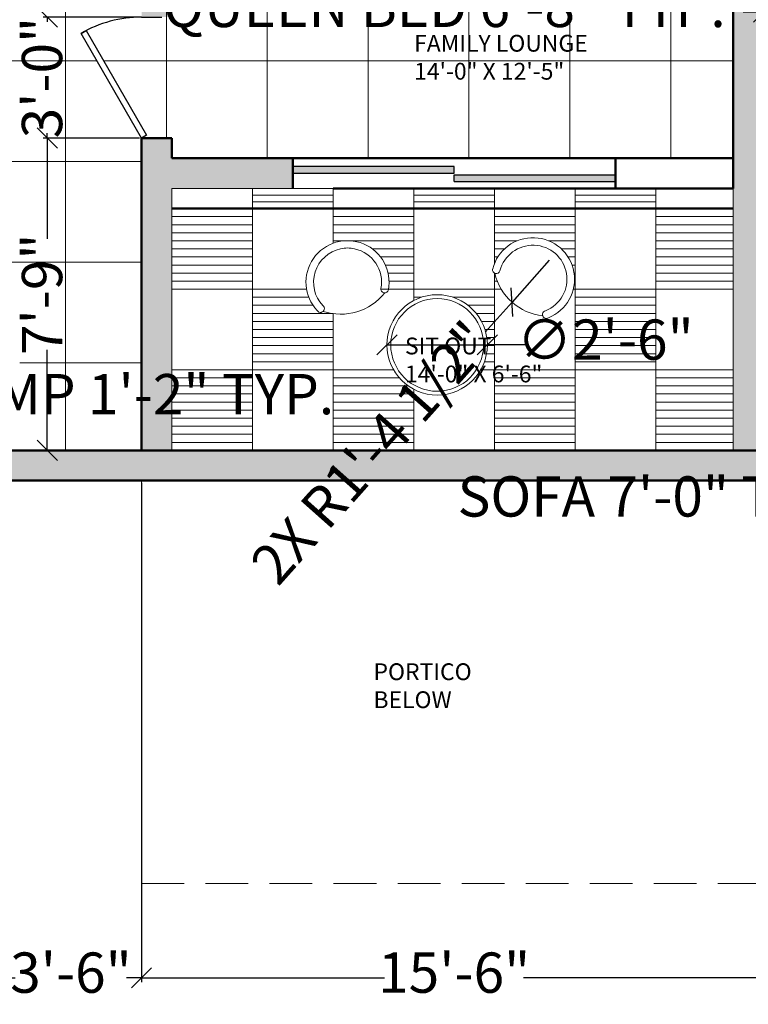
# Model space of a CAD drawing. Units: inches. Extents: x 2371 to 3019, y 129 to 700.
# Tile 2 of 14: x 2536 to 2753, y 139 to 432. Entities that reach past the tile are written whole.
import ezdxf

# ---------------------------------------------------------------- set-up
doc = ezdxf.new("R2010")
doc.units = ezdxf.units.IN
doc.linetypes.add('DASHED', pattern=[19.05, 12.7, -6.35])
for name, color, linetype, lineweight in [('A-ANNO-DIMS', 2, 'Continuous', 18), ('A-AREA-IDEN', 7, 'Continuous', 25), ('A-DOOR', 4, 'Continuous', 25), ('A-FLOR-OVHD', 20, 'DASHED', 18), ('A-FLOR-PATT', 252, 'Continuous', 13), ('A-FURN', 8, 'Continuous', 18), ('A-GLAZ', 4, 'Continuous', 25), ('A-WALL', 7, 'Continuous', 50), ('A-WALL-PATT', 8, 'Continuous', 13)]:
    doc.layers.add(name, color=color, linetype=linetype, lineweight=lineweight)
doc.styles.get("Standard").update_dxf_attribs({"font": 'arial.ttf'})
doc.dimstyles.new('ISO-25', dxfattribs={"dimtxt": 12, "dimasz": 6, "dimexe": 1.25, "dimexo": 0.625, "dimtad": 0, "dimdec": 1, "dimlunit": 3, "dimtxsty": 'Standard', "dimblk": 'OBLIQUE', "dimblk1": 'ORIGIN2', "dimblk2": 'OBLIQUE', "dimcen": 2.5, "dimadec": 0, "dimazin": 0, "dimtfac": 1, "dimtdec": 1, "dimtmove": 0, "dimatfit": 3, "dimldrblk": 'OBLIQUE', "dimfxl": 1, "dimarcsym": 0})

# ---------------------------------------------------------------- blocks, each defined once
blk = doc.blocks.new('*U4')
for p, q in [((0, 0), (0, -6)), ((36, 0), (36, -6))]:
    blk.add_line(p, q)
blk.add_lwpolyline([(0, 0), (31.18, 18), (32.05, 16.48), (0.88, -1.52)], close=True)
blk.add_arc((0, 0), 36, 0, 30)
blk = doc.blocks.new('_Oblique')
at = {"color": 0, "linetype": 'ByBlock', "lineweight": -2}
blk.add_line((-0.5, -0.5), (0.5, 0.5), dxfattribs=at)
blk = doc.blocks.new('*D20')
at = {"layer": 'A-ANNO-DIMS', "color": 0, "lineweight": -2, "transparency": 16777216}
for p, q in [((2793.86, 300.68), (2793.86, 287.46)), ((2877.86, 300.68), (2877.86, 287.46)), ((2793.86, 288.71), (2787.86, 288.71)), ((2877.86, 288.71), (2793.86, 288.71))]:
    blk.add_line(p, q, dxfattribs=at)
at = {"layer": 'Defpoints', "color": 0, "lineweight": 25, "transparency": 16777216}
for p in [(2793.86, 301.31), (2877.86, 301.31), (2793.86, 288.71)]:
    blk.add_point(p, dxfattribs=at)
at = {"layer": 'A-ANNO-DIMS', "color": 0, "lineweight": -2, "transparency": 16777216, "xscale": 6, "yscale": 6, "zscale": 6}
for p, rotation in [((2793.86, 288.71), 180.0000057391524), ((2877.86, 288.71), 5.7391524333e-06)]:
    blk.add_blockref('_Oblique', p, dxfattribs=dict(at, rotation=rotation))
at = {"layer": 'A-ANNO-DIMS', "color": 0, "transparency": 16777216, "insert": (2725.54, 288.71), "char_height": 12, "attachment_point": 5, "rotation": 0}
blk.add_mtext('SOFA 7\'-0" TYP.', dxfattribs=at)
blk = doc.blocks.new('_Origin2')
at = {"color": 0, "linetype": 'ByBlock', "lineweight": -2}
blk.add_line((-0.5, 0), (-1, 0), dxfattribs=at)
for radius in [0.5, 0.25]:
    blk.add_circle((0, 0), radius, dxfattribs=at)
blk = doc.blocks.new('*D22')
at = {"layer": 'A-ANNO-DIMS', "color": 0, "lineweight": -2, "transparency": 16777216}
for p, q in [((2432.46, 320.64), (2432.46, 317.92)), ((2446.46, 320.64), (2446.46, 317.92)), ((2432.46, 319.17), (2446.46, 319.17)), ((2446.46, 319.17), (2452.46, 319.17))]:
    blk.add_line(p, q, dxfattribs=at)
at = {"layer": 'Defpoints', "color": 0, "lineweight": 25, "transparency": 16777216}
for p in [(2432.46, 321.27), (2446.46, 321.27), (2446.46, 319.17)]:
    blk.add_point(p, dxfattribs=at)
at = {"layer": 'A-ANNO-DIMS', "color": 0, "lineweight": -2, "transparency": 16777216, "xscale": 6, "yscale": 6, "zscale": 6, "rotation": 180}
blk.add_blockref('_Oblique', (2432.46, 319.17), dxfattribs=at)
at = {"layer": 'A-ANNO-DIMS', "color": 0, "lineweight": -2, "transparency": 16777216, "xscale": 6, "yscale": 6, "zscale": 6}
blk.add_blockref('_Oblique', (2446.46, 319.17), dxfattribs=at)
at = {"layer": 'A-ANNO-DIMS', "color": 0, "transparency": 16777216, "insert": (2543.85, 319.17), "char_height": 12, "attachment_point": 5}
blk.add_mtext('TABLE LAMP 1\'-2" TYP.', dxfattribs=at)
blk = doc.blocks.new('*D24')
at = {"layer": 'A-ANNO-DIMS', "color": 0, "lineweight": -2, "transparency": 16777216}
for p, q in [((2757.61, 434.48), (2751.61, 434.48)), ((2757.61, 423.1), (2757.61, 435.73)), ((2837.61, 434.48), (2757.61, 434.48)), ((2837.61, 423.1), (2837.61, 435.73))]:
    blk.add_line(p, q, dxfattribs=at)
at = {"layer": 'Defpoints', "color": 0, "lineweight": 25, "transparency": 16777216}
for p in [(2757.61, 434.48), (2757.61, 422.48), (2837.61, 422.48)]:
    blk.add_point(p, dxfattribs=at)
at = {"layer": 'A-ANNO-DIMS', "color": 0, "lineweight": -2, "transparency": 16777216, "xscale": 6, "yscale": 6, "zscale": 6, "rotation": 180}
blk.add_blockref('_Oblique', (2757.61, 434.48), dxfattribs=at)
at = {"layer": 'A-ANNO-DIMS', "color": 0, "lineweight": -2, "transparency": 16777216, "xscale": 6, "yscale": 6, "zscale": 6}
blk.add_blockref('_Oblique', (2837.61, 434.48), dxfattribs=at)
at = {"layer": 'A-ANNO-DIMS', "color": 0, "transparency": 16777216, "insert": (2662.72, 434.48), "char_height": 12, "attachment_point": 5}
blk.add_mtext('QUEEN BED 6\'-8" TYP.', dxfattribs=at)
blk = doc.blocks.new('*D52')
at = {"layer": 'A-ANNO-DIMS', "color": 0, "lineweight": -2, "transparency": 16777216}
for p, q in [((2530.61, 294.35), (2530.61, 145.68)), ((2572.61, 294.35), (2572.61, 145.68)), ((2530.61, 146.93), (2535.03, 146.93)), ((2572.61, 146.93), (2568.18, 146.93))]:
    blk.add_line(p, q, dxfattribs=at)
at = {"layer": 'Defpoints', "color": 0, "lineweight": 25, "transparency": 16777216}
for p in [(2530.61, 294.98), (2572.61, 294.98), (2572.61, 146.93)]:
    blk.add_point(p, dxfattribs=at)
at = {"layer": 'A-ANNO-DIMS', "color": 0, "lineweight": -2, "transparency": 16777216, "xscale": 6, "yscale": 6, "zscale": 6, "rotation": 180}
blk.add_blockref('_Oblique', (2530.61, 146.93), dxfattribs=at)
at = {"layer": 'A-ANNO-DIMS', "color": 0, "lineweight": -2, "transparency": 16777216, "xscale": 6, "yscale": 6, "zscale": 6}
blk.add_blockref('_Oblique', (2572.61, 146.93), dxfattribs=at)
at = {"layer": 'A-ANNO-DIMS', "color": 0, "transparency": 16777216, "insert": (2551.61, 146.93), "char_height": 12, "attachment_point": 5}
blk.add_mtext('3\'-6"', dxfattribs=at)
blk = doc.blocks.new('*D53')
at = {"layer": 'A-ANNO-DIMS', "color": 0, "lineweight": -2, "transparency": 16777216}
for p, q in [((2572.61, 174.35), (2572.61, 145.68)), ((2758.61, 174.35), (2758.61, 145.68)), ((2572.61, 146.93), (2644.93, 146.93)), ((2758.61, 146.93), (2686.28, 146.93))]:
    blk.add_line(p, q, dxfattribs=at)
at = {"layer": 'Defpoints', "color": 0, "lineweight": 25, "transparency": 16777216}
for p in [(2572.61, 174.98), (2758.61, 174.98), (2758.61, 146.93)]:
    blk.add_point(p, dxfattribs=at)
at = {"layer": 'A-ANNO-DIMS', "color": 0, "lineweight": -2, "transparency": 16777216, "xscale": 6, "yscale": 6, "zscale": 6, "rotation": 180}
blk.add_blockref('_Oblique', (2572.61, 146.93), dxfattribs=at)
at = {"layer": 'A-ANNO-DIMS', "color": 0, "lineweight": -2, "transparency": 16777216, "xscale": 6, "yscale": 6, "zscale": 6}
blk.add_blockref('_Oblique', (2758.61, 146.93), dxfattribs=at)
at = {"layer": 'A-ANNO-DIMS', "color": 0, "transparency": 16777216, "insert": (2665.61, 146.93), "char_height": 12, "attachment_point": 5}
blk.add_mtext('15\'-6"', dxfattribs=at)
blk = doc.blocks.new('*D70')
at = {"layer": 'A-ANNO-DIMS', "color": 0, "lineweight": -2, "transparency": 16777216}
for p, q in [((2571.98, 432.98), (2543.31, 432.98)), ((2544.56, 432.98), (2544.56, 431.55)), ((2571.98, 396.98), (2543.31, 396.98)), ((2544.56, 396.98), (2544.56, 398.41))]:
    blk.add_line(p, q, dxfattribs=at)
at = {"layer": 'Defpoints', "color": 0, "lineweight": 25, "transparency": 16777216}
for p in [(2544.56, 432.98), (2572.61, 432.98), (2572.61, 396.98)]:
    blk.add_point(p, dxfattribs=at)
at = {"layer": 'A-ANNO-DIMS', "color": 0, "lineweight": -2, "transparency": 16777216, "xscale": 6, "yscale": 6, "zscale": 6}
for p, rotation in [((2544.56, 432.98), 90), ((2544.56, 396.98), 270)]:
    blk.add_blockref('_Oblique', p, dxfattribs=dict(at, rotation=rotation))
at = {"layer": 'A-ANNO-DIMS', "color": 0, "transparency": 16777216, "insert": (2544.56, 414.98), "char_height": 12, "attachment_point": 5, "rotation": 90}
blk.add_mtext('3\'-0"', dxfattribs=at)
blk = doc.blocks.new('*D71')
at = {"layer": 'A-ANNO-DIMS', "color": 0, "lineweight": -2, "transparency": 16777216}
for p, q in [((2571.98, 396.98), (2543.31, 396.98)), ((2544.56, 396.98), (2544.56, 367)), ((2544.56, 303.98), (2544.56, 333.95)), ((2571.98, 303.98), (2543.31, 303.98))]:
    blk.add_line(p, q, dxfattribs=at)
at = {"layer": 'Defpoints', "color": 0, "lineweight": 25, "transparency": 16777216}
for p in [(2544.56, 396.98), (2572.61, 396.98), (2572.61, 303.98)]:
    blk.add_point(p, dxfattribs=at)
at = {"layer": 'A-ANNO-DIMS', "color": 0, "lineweight": -2, "transparency": 16777216, "xscale": 6, "yscale": 6, "zscale": 6}
for p, rotation in [((2544.56, 396.98), 90), ((2544.56, 303.98), 270)]:
    blk.add_blockref('_Oblique', p, dxfattribs=dict(at, rotation=rotation))
at = {"layer": 'A-ANNO-DIMS', "color": 0, "transparency": 16777216, "insert": (2544.56, 350.48), "char_height": 12, "attachment_point": 5, "rotation": 90}
blk.add_mtext('7\'-9"', dxfattribs=at)
blk = doc.blocks.new('*D79')
at = {"layer": 'A-ANNO-DIMS', "color": 0, "lineweight": -2, "transparency": 16777216}
for p in [(2645.63, 335.4), (2687.48, 335.4)]:
    blk.add_line(p, (2675.48, 335.4), dxfattribs=at)
at = {"layer": 'Defpoints', "color": 0, "lineweight": 25, "transparency": 16777216}
for p in [(2645.63, 335.4), (2675.48, 335.4)]:
    blk.add_point(p, dxfattribs=at)
at = {"layer": 'A-ANNO-DIMS', "color": 0, "lineweight": -2, "transparency": 16777216, "xscale": 6, "yscale": 6, "zscale": 6}
for p, rotation in [((2645.63, 335.4), 359.9937126799771), ((2675.48, 335.4), 179.9937126799771)]:
    blk.add_blockref('_Oblique', p, dxfattribs=dict(at, rotation=rotation))
at = {"layer": 'A-ANNO-DIMS', "color": 0, "transparency": 16777216, "insert": (2710.58, 335.4), "char_height": 12, "attachment_point": 5, "rotation": 359.9937}
blk.add_mtext('∅2\'-6"', dxfattribs=at)
blk = doc.blocks.new('*D80')
at = {"layer": 'A-ANNO-DIMS', "color": 0, "lineweight": -2, "transparency": 16777216}
for p in [(2693.9, 360.58), (2674.84, 339.15)]:
    blk.add_line(p, (2682.82, 348.12), dxfattribs=at)
at = {"layer": 'Defpoints', "color": 0, "lineweight": 25, "transparency": 16777216}
for p in [(2693.9, 360.58), (2682.82, 348.12)]:
    blk.add_point(p, dxfattribs=at)
at = {"layer": 'A-ANNO-DIMS', "color": 0, "lineweight": -2, "transparency": 16777216, "xscale": 6, "yscale": 6, "zscale": 6, "rotation": 48.3550235308778}
blk.add_blockref('_Oblique', (2682.82, 348.12), dxfattribs=at)
at = {"layer": 'A-ANNO-DIMS', "color": 0, "transparency": 16777216, "insert": (2642.09, 302.32), "char_height": 12, "attachment_point": 5, "rotation": 48.355}
blk.add_mtext('2X R1\'-4 1/2"', dxfattribs=at)

msp = doc.modelspace()

# ---------------------------------------------------------------- hatches: boundary and pattern name
at = {"layer": 'A-FLOR-PATT'}
h = msp.add_hatch(dxfattribs=at)
h.set_pattern_fill('_USER', color=256, scale=30, pattern_type=0)
h.set_pattern_definition([(0, (0, 0), (0, 30), [])])
h.paths.add_polyline_path([(2913.11, 498.98), (2827.61, 498.98), (2827.61, 531.98), (2832.11, 531.98), (2832.11, 537.98), (2833.61, 537.98), (2833.61, 605.98), (2818.35, 605.98, -1), (2796.86, 605.98), (2781.61, 605.98), (2781.61, 603.98), (2781.61, 533.98), (2757.61, 533.98), (2757.61, 531.98), (2797.61, 531.98), (2797.61, 522.98), (2757.61, 522.98), (2757.61, 516.98), (2754.59, 516.98), (2772.52, 485.76), (2771.01, 484.89), (2770.98, 484.93, -0.097552), (2757.61, 481.1), (2757.61, 422.48), (2837.61, 422.48), (2837.61, 362.48), (2757.61, 362.48), (2757.61, 303.98), (2835.86, 303.98, -0.09439), (2793.86, 311.98), (2793.86, 337.98), (2799.86, 337.98), (2799.86, 336.42), (2871.86, 336.42), (2871.86, 337.98), (2877.86, 337.98), (2877.86, 311.98, -0.09439), (2835.86, 303.98), (2913.11, 303.98), (2913.11, 383.18), (2904.11, 383.18), (2904.11, 419.18), (2913.11, 419.18)])
h.paths.add_polyline_path([(2788.88, 332.88), (2788.88, 308.88), (2764.88, 308.88), (2764.88, 332.88)], flags=16)
h.paths.add_polyline_path([(2788.4, 325.04, -1), (2774.4, 325.04, -1)], flags=0)
h.paths.add_polyline_path([(2781.4, 328.04), (2784.4, 325.04), (2781.4, 322.04), (2778.4, 325.04)], flags=0)
h.paths.add_polyline_path([(2782.4, 325.04, -1), (2780.4, 325.04, -1)], flags=0)
h.paths.add_polyline_path([(2748.61, 480.99), (2754.51, 480.98, 0.119303), (2770.98, 484.93), (2753.07, 516.1), (2754.59, 516.98), (2748.61, 516.98), (2748.61, 539.98), (2712.61, 539.98), (2665.11, 539.98, -0.09439), (2707.11, 531.98), (2707.11, 505.98), (2701.11, 505.98), (2701.11, 507.53), (2629.11, 507.53), (2629.11, 505.98), (2623.11, 505.98), (2623.11, 531.98, -0.09439), (2665.11, 539.98), (2581.61, 539.98), (2581.61, 522.98), (2581.61, 477.98, -0.131044), (2589.61, 507.98), (2615.61, 507.98), (2615.61, 501.98), (2614.05, 501.98), (2614.05, 453.98), (2615.61, 453.98), (2615.61, 447.98), (2589.61, 447.98, -0.131044), (2581.61, 477.98), (2581.61, 432.98), (2572.61, 432.98, 0.119303), (2556.14, 428.99), (2574.12, 397.85), (2572.61, 396.98), (2578.61, 396.98), (2581.61, 396.98), (2581.61, 390.98), (2748.61, 390.98)])
h.paths.add_polyline_path([(2683.1, 447.25), (2652.43, 447.25), (2652.43, 492.22), (2683.1, 492.22)], flags=16)
h.paths.add_polyline_path([(2682.1, 448.25), (2653.43, 448.25), (2653.43, 491.22), (2682.1, 491.22)], flags=0)
h.paths.add_polyline_path([(2613.58, 512.06), (2589.58, 512.06), (2589.58, 536.06), (2613.58, 536.06)], flags=16)
h.paths.add_polyline_path([(2599.1, 528.22, -1), (2613.1, 528.22, -1)], flags=0)
h.paths.add_polyline_path([(2609.1, 528.22), (2606.1, 525.22), (2603.1, 528.22), (2606.1, 531.22)], flags=0)
h.paths.add_polyline_path([(2607.1, 528.22, -1), (2605.1, 528.22, -1)], flags=0)
h.paths.add_polyline_path([(2581.61, 522.98), (2581.61, 621.98), (2572.61, 621.98), (2572.61, 522.98), (2572.61, 500.98), (2565.85, 500.98), (2565.85, 500.15), (2564.82, 500.15), (2561.16, 500.19), (2561.16, 500.17), (2560.13, 500.3), (2560.22, 500.98), (2556.38, 500.98), (2556.43, 500.22), (2555.4, 500.14), (2555.34, 500.98), (2551.07, 500.98), (2551.07, 500.15), (2550.04, 500.15), (2547.64, 500.19), (2547.64, 500.15), (2546.61, 500.15), (2541.79, 500.22), (2540.72, 500.13), (2540.65, 500.98), (2533.37, 500.98), (2533.37, 500.15), (2532.34, 500.15), (2529.13, 500.21), (2529.12, 500.13), (2528.09, 500.22), (2528.16, 500.98), (2523.23, 500.98), (2523.23, 500.15), (2522.2, 500.15), (2519.8, 500.21), (2519.8, 500.15), (2518.77, 500.15), (2514.45, 500.26), (2514.44, 500.14), (2513.41, 500.22), (2513.47, 500.98), (2509.62, 500.98), (2509.71, 500.3), (2508.69, 500.17), (2508.58, 500.98), (2505.03, 500.98), (2505.03, 500.15), (2503.99, 500.15), (2501.07, 500.29), (2501.07, 500.15), (2500.04, 500.15), (2496.44, 500.37), (2496.44, 500.15), (2495.4, 500.15), (2492.55, 500.41), (2492.18, 500.35), (2492.09, 500.98), (2486.11, 500.98), (2486.11, 524.98), (2486.11, 531.98), (2490.61, 531.98), (2490.61, 537.98), (2492.11, 537.98), (2492.11, 605.98), (2476.85, 605.98, -1), (2455.36, 605.98), (2440.11, 605.98), (2440.11, 533.98), (2416.11, 533.98), (2416.11, 605.98), (2416.11, 621.98), (2536.61, 621.98), (2536.61, 630.98), (2407.11, 630.98), (2407.11, 363.98), (2416.11, 363.98), (2416.11, 431.48), (2496.11, 431.48), (2496.11, 371.48), (2416.11, 371.48), (2416.11, 303.98), (2494.36, 303.98, -0.09439), (2452.36, 311.98), (2452.36, 337.98), (2458.36, 337.98), (2458.36, 336.42), (2530.36, 336.42), (2530.36, 337.98), (2536.36, 337.98), (2536.36, 311.98, -0.09439), (2494.36, 303.98), (2572.61, 303.98), (2572.61, 381.98), (2572.61, 396.98), (2554.61, 428.15), (2556.12, 429.03), (2556.14, 428.99, -0.119303), (2572.61, 432.98), (2578.61, 432.98), (2581.61, 432.98)])
h.paths.add_polyline_path([(2450.11, 500.98), (2444.5, 500.98), (2444.44, 500.14), (2443.41, 500.22), (2443.47, 500.98), (2439.62, 500.98), (2439.71, 500.3), (2438.69, 500.17), (2438.58, 500.98), (2435.02, 500.98), (2435.02, 500.15), (2433.99, 500.15), (2433.99, 500.98), (2431.07, 500.98), (2431.07, 500.15), (2430.04, 500.15), (2430.04, 500.98), (2426.43, 500.98), (2426.43, 500.15), (2425.4, 500.15), (2425.4, 500.98), (2423.13, 500.98), (2423.2, 500.5), (2422.18, 500.35), (2422.09, 500.98), (2416.11, 500.98), (2416.11, 524.98), (2416.11, 531.98), (2450.11, 531.98), (2450.11, 522.98)], flags=16)
h.paths.add_polyline_path([(2449.11, 501.98), (2417.11, 501.98), (2417.11, 522.98), (2417.11, 523.98), (2449.11, 523.98)], flags=0)
h.paths.add_polyline_path([(2420.7, 510.73), (2419.36, 520.07), (2420.38, 520.22), (2421.74, 510.73), (2425.4, 510.73), (2425.4, 520.07), (2426.43, 520.07), (2426.43, 510.73), (2430.04, 510.73), (2430.04, 520.07), (2431.07, 520.07), (2431.07, 510.73), (2433.99, 510.73), (2433.99, 520.07), (2435.02, 520.07), (2435.02, 510.73), (2437.35, 510.73), (2436.18, 519.93), (2437.2, 520.06), (2438.39, 510.73), (2444.17, 510.73), (2444.85, 520.08), (2445.88, 520.01), (2445.21, 510.73)], flags=0)
h.paths.add_polyline_path([(2446.94, 336.11), (2446.94, 312.11), (2422.94, 312.11), (2422.94, 336.11)], flags=16)
h.paths.add_polyline_path([(2446.46, 328.27, -1), (2432.46, 328.27, -1)], flags=0)
h.paths.add_polyline_path([(2439.46, 331.27), (2442.46, 328.27), (2439.46, 325.27), (2436.46, 328.27)], flags=0)
h.paths.add_polyline_path([(2440.46, 328.27, -1), (2438.46, 328.27, -1)], flags=0)
h.paths.add_polyline_path([(2816, 444.88), (2866.87, 444.88), (2866.87, 463.54), (2816, 463.54)], flags=24)
h.paths.add_polyline_path([(2794.21, 558.3), (2833.34, 558.3), (2833.34, 576.96), (2794.21, 576.96)], flags=24)
h.paths.add_polyline_path([(2651.69, 411.53), (2711.04, 411.53), (2711.04, 430.19), (2651.69, 430.19)], flags=24)
h.paths.add_polyline_path([(2494.09, 444.88), (2544.97, 444.88), (2544.97, 463.54), (2494.09, 463.54)], flags=24)
h.paths.add_polyline_path([(2444.55, 565.02), (2483.69, 565.02), (2483.69, 583.68), (2444.55, 583.68)], flags=24)
h = msp.add_hatch(dxfattribs=at)
h.set_pattern_fill('_USER', color=256, scale=30, angle=90, pattern_type=0)
h.set_pattern_definition([(90, (0, 0), (-30, 2e-15), [])])
h.paths.add_polyline_path([(2913.11, 498.98), (2827.61, 498.98), (2827.61, 531.98), (2832.11, 531.98), (2832.11, 537.98), (2833.61, 537.98), (2833.61, 605.98), (2818.35, 605.98, -1), (2796.86, 605.98), (2781.61, 605.98), (2781.61, 603.98), (2781.61, 533.98), (2757.61, 533.98), (2757.61, 531.98), (2797.61, 531.98), (2797.61, 522.98), (2757.61, 522.98), (2757.61, 516.98), (2754.59, 516.98), (2772.52, 485.76), (2771.01, 484.89), (2770.98, 484.93, -0.097552), (2757.61, 481.1), (2757.61, 422.48), (2837.61, 422.48), (2837.61, 362.48), (2757.61, 362.48), (2757.61, 303.98), (2835.86, 303.98, -0.09439), (2793.86, 311.98), (2793.86, 337.98), (2799.86, 337.98), (2799.86, 336.42), (2871.86, 336.42), (2871.86, 337.98), (2877.86, 337.98), (2877.86, 311.98, -0.09439), (2835.86, 303.98), (2913.11, 303.98), (2913.11, 383.18), (2904.11, 383.18), (2904.11, 419.18), (2913.11, 419.18)])
h.paths.add_polyline_path([(2788.88, 332.88), (2788.88, 308.88), (2764.88, 308.88), (2764.88, 332.88)], flags=16)
h.paths.add_polyline_path([(2788.4, 325.04, -1), (2774.4, 325.04, -1)], flags=0)
h.paths.add_polyline_path([(2781.4, 328.04), (2784.4, 325.04), (2781.4, 322.04), (2778.4, 325.04)], flags=0)
h.paths.add_polyline_path([(2782.4, 325.04, -1), (2780.4, 325.04, -1)], flags=0)
h.paths.add_polyline_path([(2748.61, 480.99), (2754.51, 480.98, 0.119303), (2770.98, 484.93), (2753.07, 516.1), (2754.59, 516.98), (2748.61, 516.98), (2748.61, 539.98), (2712.61, 539.98), (2665.11, 539.98, -0.09439), (2707.11, 531.98), (2707.11, 505.98), (2701.11, 505.98), (2701.11, 507.53), (2629.11, 507.53), (2629.11, 505.98), (2623.11, 505.98), (2623.11, 531.98, -0.09439), (2665.11, 539.98), (2581.61, 539.98), (2581.61, 522.98), (2581.61, 477.98, -0.131044), (2589.61, 507.98), (2615.61, 507.98), (2615.61, 501.98), (2614.05, 501.98), (2614.05, 453.98), (2615.61, 453.98), (2615.61, 447.98), (2589.61, 447.98, -0.131044), (2581.61, 477.98), (2581.61, 432.98), (2572.61, 432.98, 0.119303), (2556.14, 428.99), (2574.12, 397.85), (2572.61, 396.98), (2578.61, 396.98), (2581.61, 396.98), (2581.61, 390.98), (2748.61, 390.98)])
h.paths.add_polyline_path([(2683.1, 447.25), (2652.43, 447.25), (2652.43, 492.22), (2683.1, 492.22)], flags=16)
h.paths.add_polyline_path([(2682.1, 448.25), (2653.43, 448.25), (2653.43, 491.22), (2682.1, 491.22)], flags=0)
h.paths.add_polyline_path([(2613.58, 512.06), (2589.58, 512.06), (2589.58, 536.06), (2613.58, 536.06)], flags=16)
h.paths.add_polyline_path([(2599.1, 528.22, -1), (2613.1, 528.22, -1)], flags=0)
h.paths.add_polyline_path([(2609.1, 528.22), (2606.1, 525.22), (2603.1, 528.22), (2606.1, 531.22)], flags=0)
h.paths.add_polyline_path([(2607.1, 528.22, -1), (2605.1, 528.22, -1)], flags=0)
h.paths.add_polyline_path([(2581.61, 522.98), (2581.61, 621.98), (2572.61, 621.98), (2572.61, 522.98), (2572.61, 500.98), (2565.85, 500.98), (2565.85, 500.15), (2564.82, 500.15), (2561.16, 500.19), (2561.16, 500.17), (2560.13, 500.3), (2560.22, 500.98), (2556.38, 500.98), (2556.43, 500.22), (2555.4, 500.14), (2555.34, 500.98), (2551.07, 500.98), (2551.07, 500.15), (2550.04, 500.15), (2547.64, 500.19), (2547.64, 500.15), (2546.61, 500.15), (2541.79, 500.22), (2540.72, 500.13), (2540.65, 500.98), (2533.37, 500.98), (2533.37, 500.15), (2532.34, 500.15), (2529.13, 500.21), (2529.12, 500.13), (2528.09, 500.22), (2528.16, 500.98), (2523.23, 500.98), (2523.23, 500.15), (2522.2, 500.15), (2519.8, 500.21), (2519.8, 500.15), (2518.77, 500.15), (2514.45, 500.26), (2514.44, 500.14), (2513.41, 500.22), (2513.47, 500.98), (2509.62, 500.98), (2509.71, 500.3), (2508.69, 500.17), (2508.58, 500.98), (2505.03, 500.98), (2505.03, 500.15), (2503.99, 500.15), (2501.07, 500.29), (2501.07, 500.15), (2500.04, 500.15), (2496.44, 500.37), (2496.44, 500.15), (2495.4, 500.15), (2492.55, 500.41), (2492.18, 500.35), (2492.09, 500.98), (2486.11, 500.98), (2486.11, 524.98), (2486.11, 531.98), (2490.61, 531.98), (2490.61, 537.98), (2492.11, 537.98), (2492.11, 605.98), (2476.85, 605.98, -1), (2455.36, 605.98), (2440.11, 605.98), (2440.11, 533.98), (2416.11, 533.98), (2416.11, 605.98), (2416.11, 621.98), (2536.61, 621.98), (2536.61, 630.98), (2407.11, 630.98), (2407.11, 363.98), (2416.11, 363.98), (2416.11, 431.48), (2496.11, 431.48), (2496.11, 371.48), (2416.11, 371.48), (2416.11, 303.98), (2494.36, 303.98, -0.09439), (2452.36, 311.98), (2452.36, 337.98), (2458.36, 337.98), (2458.36, 336.42), (2530.36, 336.42), (2530.36, 337.98), (2536.36, 337.98), (2536.36, 311.98, -0.09439), (2494.36, 303.98), (2572.61, 303.98), (2572.61, 381.98), (2572.61, 396.98), (2554.61, 428.15), (2556.12, 429.03), (2556.14, 428.99, -0.119303), (2572.61, 432.98), (2578.61, 432.98), (2581.61, 432.98)])
h.paths.add_polyline_path([(2450.11, 500.98), (2444.5, 500.98), (2444.44, 500.14), (2443.41, 500.22), (2443.47, 500.98), (2439.62, 500.98), (2439.71, 500.3), (2438.69, 500.17), (2438.58, 500.98), (2435.02, 500.98), (2435.02, 500.15), (2433.99, 500.15), (2433.99, 500.98), (2431.07, 500.98), (2431.07, 500.15), (2430.04, 500.15), (2430.04, 500.98), (2426.43, 500.98), (2426.43, 500.15), (2425.4, 500.15), (2425.4, 500.98), (2423.13, 500.98), (2423.2, 500.5), (2422.18, 500.35), (2422.09, 500.98), (2416.11, 500.98), (2416.11, 524.98), (2416.11, 531.98), (2450.11, 531.98), (2450.11, 522.98)], flags=16)
h.paths.add_polyline_path([(2449.11, 501.98), (2417.11, 501.98), (2417.11, 522.98), (2417.11, 523.98), (2449.11, 523.98)], flags=0)
h.paths.add_polyline_path([(2420.7, 510.73), (2419.36, 520.07), (2420.38, 520.22), (2421.74, 510.73), (2425.4, 510.73), (2425.4, 520.07), (2426.43, 520.07), (2426.43, 510.73), (2430.04, 510.73), (2430.04, 520.07), (2431.07, 520.07), (2431.07, 510.73), (2433.99, 510.73), (2433.99, 520.07), (2435.02, 520.07), (2435.02, 510.73), (2437.35, 510.73), (2436.18, 519.93), (2437.2, 520.06), (2438.39, 510.73), (2444.17, 510.73), (2444.85, 520.08), (2445.88, 520.01), (2445.21, 510.73)], flags=0)
h.paths.add_polyline_path([(2446.94, 336.11), (2446.94, 312.11), (2422.94, 312.11), (2422.94, 336.11)], flags=16)
h.paths.add_polyline_path([(2446.46, 328.27, -1), (2432.46, 328.27, -1)], flags=0)
h.paths.add_polyline_path([(2439.46, 331.27), (2442.46, 328.27), (2439.46, 325.27), (2436.46, 328.27)], flags=0)
h.paths.add_polyline_path([(2440.46, 328.27, -1), (2438.46, 328.27, -1)], flags=0)
h.paths.add_polyline_path([(2816, 444.88), (2866.87, 444.88), (2866.87, 463.54), (2816, 463.54)], flags=24)
h.paths.add_polyline_path([(2794.21, 558.3), (2833.34, 558.3), (2833.34, 576.96), (2794.21, 576.96)], flags=24)
h.paths.add_polyline_path([(2651.69, 411.53), (2711.04, 411.53), (2711.04, 430.19), (2651.69, 430.19)], flags=24)
h.paths.add_polyline_path([(2494.09, 444.88), (2544.97, 444.88), (2544.97, 463.54), (2494.09, 463.54)], flags=24)
h.paths.add_polyline_path([(2444.55, 565.02), (2483.69, 565.02), (2483.69, 583.68), (2444.55, 583.68)], flags=24)
at = {"layer": 'A-GLAZ'}
h = msp.add_hatch(color=256, dxfattribs=at)
h.dxf.hatch_style = 1
h.paths.add_polyline_path([(2665.61, 388.48), (2617.61, 388.48), (2617.61, 386.48), (2665.61, 386.48)])
h.paths.add_polyline_path([(2713.61, 386.05), (2665.61, 386.05), (2665.61, 384.05), (2713.61, 384.05)])
at = {"layer": 'A-WALL-PATT'}
h = msp.add_hatch(color=256, dxfattribs=at)
h.dxf.hatch_style = 1
h.paths.add_polyline_path([(2536.61, 630.98), (2407.11, 630.98), (2407.11, 363.98), (2416.11, 363.98), (2416.11, 498.98), (2416.11, 522.98), (2416.11, 531.98), (2416.11, 603.98), (2416.11, 621.98), (2536.61, 621.98)])
h.paths.add_polyline_path([(2630.98, 630.98), (2560.61, 630.98), (2560.61, 621.98), (2630.98, 621.98)])
h.paths.add_polyline_path([(2878.11, 630.98), (2699.23, 630.98), (2699.23, 621.98), (2878.11, 621.98)])
h.paths.add_polyline_path([(2496.61, 621.98), (2492.11, 621.98), (2492.11, 569.98), (2496.61, 569.98)], flags=17)
h.paths.add_polyline_path([(2581.61, 621.98), (2572.61, 621.98), (2572.61, 522.98), (2572.61, 498.98), (2572.61, 432.98), (2578.61, 432.98), (2581.61, 432.98), (2581.61, 522.98)])
h.paths.add_polyline_path([(2572.61, 531.98), (2486.11, 531.98), (2486.11, 522.98), (2572.61, 522.98)])
h.paths.add_polyline_path([(2450.11, 531.98), (2440.11, 531.98), (2416.11, 531.98), (2416.11, 522.98), (2450.11, 522.98)], flags=17)
h.paths.add_polyline_path([(2416.11, 315.98), (2407.11, 315.98), (2407.11, 294.98), (2458.11, 294.98), (2458.11, 303.98), (2416.11, 303.98)])
h.paths.add_polyline_path([(2757.61, 303.98), (2530.61, 303.98), (2530.61, 294.98), (2757.61, 294.98)])
h.paths.add_polyline_path([(2581.61, 381.98), (2605.61, 381.98), (2617.61, 381.98), (2617.61, 390.98), (2581.61, 390.98), (2581.61, 396.98), (2572.61, 396.98), (2572.61, 381.98), (2572.61, 303.98), (2581.61, 303.98)])
h.paths.add_polyline_path([(2757.61, 480.98), (2748.61, 480.98), (2748.61, 381.98), (2748.61, 303.98), (2757.61, 303.98), (2757.61, 381.98), (2757.61, 422.48)])
h.paths.add_polyline_path([(2797.61, 531.98), (2757.61, 531.98), (2757.61, 603.98), (2757.61, 621.98), (2748.61, 621.98), (2748.61, 516.99), (2754.59, 516.98), (2757.61, 516.98), (2757.61, 522.98), (2797.61, 522.98)])
h.paths.add_polyline_path([(2913.11, 531.98), (2827.61, 531.98), (2827.61, 522.98), (2913.11, 522.98)])
h.paths.add_polyline_path([(2923.11, 630.98), (2902.11, 630.98), (2902.11, 621.98), (2914.11, 621.98), (2914.11, 363.98), (2923.11, 363.98)])
h.paths.add_polyline_path([(2923.11, 315.98), (2914.11, 315.98), (2914.11, 303.98), (2866.11, 303.98), (2866.11, 294.98), (2923.11, 294.98)])
h.paths.add_polyline_path([(2793.61, 303.98), (2757.61, 303.98), (2757.61, 294.98), (2793.61, 294.98)])

# ---------------------------------------------------------------- linework, layer by layer
at = {"layer": 'A-FLOR-OVHD'}
msp.add_lwpolyline([(2572.61, 294.98), (2572.61, 174.98), (2758.61, 174.98), (2758.61, 294.98)], dxfattribs=at)
at = {"layer": 'A-FLOR-PATT'}
for p, q in [((2581.61, 381.98), (2581.61, 303.98)), ((2581.61, 381.98), (2605.61, 381.98)), ((2605.61, 381.98), (2605.61, 303.98)), ((2605.61, 381.98), (2629.61, 381.98)), ((2629.61, 381.98), (2629.61, 365.67)), ((2653.61, 381.98), (2653.61, 348.61)), ((2653.61, 381.98), (2677.61, 381.98)), ((2677.61, 381.98), (2677.61, 359.63)), ((2701.61, 381.98), (2701.61, 303.98)), ((2701.61, 381.98), (2725.61, 381.98)), ((2725.61, 381.98), (2725.61, 303.98)), ((2748.61, 303.98), (2748.61, 381.98)), ((2605.61, 379.98), (2629.61, 379.98)), ((2653.61, 379.98), (2677.61, 379.98)), ((2701.61, 379.98), (2725.61, 379.98)), ((2581.61, 375.98), (2605.61, 375.98)), ((2605.61, 377.98), (2629.61, 377.98)), ((2605.61, 375.98), (2629.61, 375.98)), ((2629.61, 375.98), (2653.61, 375.98)), ((2653.61, 377.98), (2677.61, 377.98)), ((2653.61, 375.98), (2677.61, 375.98)), ((2677.61, 375.98), (2701.61, 375.98)), ((2701.61, 377.98), (2725.61, 377.98)), ((2701.61, 375.98), (2725.61, 375.98)), ((2725.61, 375.98), (2748.61, 375.98)), ((2581.61, 373.58), (2605.61, 373.58)), ((2629.61, 373.58), (2653.61, 373.58)), ((2677.61, 373.58), (2701.61, 373.58)), ((2725.61, 373.58), (2748.61, 373.58)), ((2581.61, 371.18), (2605.61, 371.18)), ((2629.61, 371.18), (2653.61, 371.18)), ((2677.61, 371.18), (2701.61, 371.18)), ((2725.61, 371.18), (2748.61, 371.18)), ((2581.61, 368.78), (2605.61, 368.78)), ((2629.61, 368.78), (2653.61, 368.78)), ((2677.61, 368.78), (2701.61, 368.78)), ((2725.61, 368.78), (2748.61, 368.78)), ((2581.61, 366.38), (2605.61, 366.38)), ((2581.61, 363.98), (2605.61, 363.98)), ((2629.61, 366.38), (2653.61, 366.38)), ((2641.28, 363.98), (2653.61, 363.98)), ((2677.61, 366.38), (2684.32, 366.38)), ((2677.61, 363.98), (2680.6, 363.98)), ((2693.77, 366.38), (2701.61, 366.38)), ((2697.5, 363.98), (2701.61, 363.98)), ((2725.61, 366.38), (2748.61, 366.38)), ((2725.61, 363.98), (2748.61, 363.98)), ((2581.61, 361.58), (2605.61, 361.58)), ((2643.71, 361.58), (2653.61, 361.58)), ((2677.61, 361.58), (2678.61, 361.58)), ((2699.48, 361.58), (2701.61, 361.58)), ((2725.61, 361.58), (2748.61, 361.58)), ((2581.61, 359.18), (2605.61, 359.18)), ((2645.15, 359.18), (2653.61, 359.18)), ((2700.66, 359.18), (2701.61, 359.18)), ((2725.61, 359.18), (2748.61, 359.18)), ((2581.61, 356.78), (2605.61, 356.78)), ((2645.95, 356.78), (2653.61, 356.78)), ((2677.61, 356.78), (2677.61, 303.98)), ((2701.27, 356.78), (2701.61, 356.78)), ((2725.61, 356.78), (2748.61, 356.78)), ((2581.61, 354.38), (2605.61, 354.38)), ((2581.61, 351.98), (2621.71, 351.98)), ((2581.61, 351.98), (2605.61, 351.98)), ((2605.61, 351.98), (2621.71, 351.98)), ((2643.82, 351.98), (2679.62, 351.98)), ((2646.07, 351.98), (2653.61, 351.98)), ((2646.24, 354.38), (2653.61, 354.38)), ((2653.61, 351.98), (2677.61, 351.98)), ((2677.61, 354.38), (2678.42, 354.38)), ((2677.61, 351.98), (2679.62, 351.98)), ((2701.04, 351.98), (2748.61, 351.98)), ((2701.04, 351.98), (2701.61, 351.98)), ((2701.39, 354.38), (2701.61, 354.38)), ((2701.61, 351.98), (2725.61, 351.98)), ((2725.61, 354.38), (2748.61, 354.38)), ((2725.61, 351.98), (2748.61, 351.98)), ((2605.61, 349.58), (2622.38, 349.58)), ((2653.61, 349.58), (2655.87, 349.58)), ((2665.23, 349.58), (2677.61, 349.58)), ((2701.61, 349.58), (2725.61, 349.58)), ((2605.61, 347.18), (2623.63, 347.18)), ((2669.73, 347.18), (2677.61, 347.18)), ((2701.61, 347.18), (2725.61, 347.18)), ((2605.61, 344.78), (2629.61, 344.78)), ((2629.61, 344.78), (2629.61, 303.98)), ((2672.17, 344.78), (2677.61, 344.78)), ((2701.61, 344.78), (2725.61, 344.78)), ((2605.61, 342.38), (2629.61, 342.38)), ((2673.75, 342.38), (2677.61, 342.38)), ((2701.61, 342.38), (2725.61, 342.38)), ((2605.61, 339.98), (2629.61, 339.98)), ((2605.61, 337.58), (2629.61, 337.58)), ((2674.76, 339.98), (2677.61, 339.98)), ((2675.32, 337.58), (2677.61, 337.58)), ((2701.61, 339.98), (2725.61, 339.98)), ((2701.61, 337.58), (2725.61, 337.58)), ((2605.61, 335.18), (2629.61, 335.18)), ((2675.48, 335.18), (2677.61, 335.18)), ((2701.61, 335.18), (2725.61, 335.18)), ((2605.61, 332.78), (2629.61, 332.78)), ((2675.25, 332.78), (2677.61, 332.78)), ((2701.61, 332.78), (2725.61, 332.78)), ((2605.61, 330.38), (2629.61, 330.38)), ((2674.61, 330.38), (2677.61, 330.38)), ((2701.61, 330.38), (2725.61, 330.38)), ((2581.61, 327.98), (2647.6, 327.98)), ((2581.61, 327.98), (2605.61, 327.98)), ((2581.61, 325.58), (2605.61, 325.58)), ((2605.61, 327.98), (2629.61, 327.98)), ((2629.61, 327.98), (2647.6, 327.98)), ((2629.61, 325.58), (2649.32, 325.58)), ((2673.5, 327.98), (2677.61, 327.98)), ((2673.5, 327.98), (2748.61, 327.98)), ((2677.61, 327.98), (2701.61, 327.98)), ((2677.61, 325.58), (2701.61, 325.58)), ((2701.61, 327.98), (2725.61, 327.98)), ((2725.61, 327.98), (2748.61, 327.98)), ((2725.61, 325.58), (2748.61, 325.58)), ((2581.61, 323.18), (2605.61, 323.18)), ((2629.61, 323.18), (2651.99, 323.18)), ((2677.61, 323.18), (2701.61, 323.18)), ((2725.61, 323.18), (2748.61, 323.18)), ((2581.61, 320.78), (2605.61, 320.78)), ((2629.61, 320.78), (2653.61, 320.78)), ((2653.61, 322.19), (2653.61, 303.98)), ((2677.61, 320.78), (2701.61, 320.78)), ((2725.61, 320.78), (2748.61, 320.78)), ((2581.61, 318.38), (2605.61, 318.38)), ((2629.61, 318.38), (2653.61, 318.38)), ((2677.61, 318.38), (2701.61, 318.38)), ((2725.61, 318.38), (2748.61, 318.38)), ((2581.61, 315.98), (2605.61, 315.98)), ((2629.61, 315.98), (2653.61, 315.98)), ((2677.61, 315.98), (2701.61, 315.98)), ((2725.61, 315.98), (2748.61, 315.98)), ((2581.61, 313.58), (2605.61, 313.58)), ((2581.61, 311.18), (2605.61, 311.18)), ((2629.61, 313.58), (2653.61, 313.58)), ((2629.61, 311.18), (2653.61, 311.18)), ((2677.61, 313.58), (2701.61, 313.58)), ((2677.61, 311.18), (2701.61, 311.18)), ((2725.61, 313.58), (2748.61, 313.58)), ((2725.61, 311.18), (2748.61, 311.18)), ((2581.61, 308.78), (2605.61, 308.78)), ((2629.61, 308.78), (2653.61, 308.78)), ((2677.61, 308.78), (2701.61, 308.78)), ((2725.61, 308.78), (2748.61, 308.78)), ((2581.61, 306.38), (2605.61, 306.38)), ((2629.61, 306.38), (2653.61, 306.38)), ((2677.61, 306.38), (2701.61, 306.38)), ((2725.61, 306.38), (2748.61, 306.38))]:
    msp.add_line(p, q, dxfattribs=at)
at = {"layer": 'A-FURN'}
for radius in [14.93, 13.81]:
    msp.add_circle((2660.55, 335.4), radius, dxfattribs=at)
for centre, radius, start, end in [((2689.05, 354.96), 12.36, 291.8077, 165.7864), ((2633.89, 354.07), 12.36, 349.261, 223.2397), ((2633.89, 354.07), 10.12, 101.8695, 223.2397), ((2633.89, 356.35), 7.9, 74.7317, 105.2683), ((2633.89, 354.07), 10.12, 349.261, 78.1305), ((2689.05, 354.96), 10.12, 291.8077, 165.7864), ((2678.15, 357.73), 1.12, 166.4865, 345.0864), ((2693.9, 360.58), 16.68, 193.4052, 263.3042), ((2644.93, 351.99), 1.12, 169.961, 348.5609), ((2631.86, 361.22), 16.68, 251.7432, 321.6422), ((2625.85, 346.21), 1.14, 212.1648, 54.3145), ((2693.02, 344.44), 1.14, 100.7329, 302.8826)]:
    msp.add_arc(centre, radius, start, end, dxfattribs=at)
at = {"layer": 'A-GLAZ'}
for p, q in [((2665.61, 388.48), (2617.61, 388.48)), ((2665.61, 386.48), (2665.61, 388.48)), ((2617.61, 386.48), (2665.61, 386.48)), ((2665.61, 386.05), (2713.61, 386.05)), ((2665.61, 384.05), (2665.61, 386.05)), ((2665.61, 384.05), (2713.61, 384.05))]:
    msp.add_line(p, q, dxfattribs=at)
at = {"layer": 'A-WALL'}
for p, q in [((2748.61, 381.98), (2748.61, 480.98)), ((2572.61, 396.98), (2581.61, 396.98)), ((2572.61, 396.98), (2572.61, 381.98)), ((2581.61, 396.98), (2581.61, 390.98)), ((2581.61, 390.98), (2748.61, 390.98)), ((2617.61, 390.98), (2617.61, 381.98)), ((2713.61, 390.98), (2713.61, 381.98)), ((2572.61, 381.98), (2572.61, 303.98)), ((2629.61, 381.98), (2748.61, 381.98)), ((2581.61, 375.98), (2748.61, 375.98)), ((2416.11, 303.98), (2914.11, 303.98)), ((2581.61, 303.98), (2605.61, 303.98)), ((2629.61, 303.98), (2653.61, 303.98)), ((2677.61, 303.98), (2701.61, 303.98)), ((2725.61, 303.98), (2748.61, 303.98)), ((2407.11, 294.98), (2923.11, 294.98))]:
    msp.add_line(p, q, dxfattribs=at)

# ---------------------------------------------------------------- block references
at = {"layer": 'A-DOOR', "rotation": 90}
msp.add_blockref('*U4', (2572.61, 396.98), dxfattribs=at)

# ---------------------------------------------------------------- texts
at = {"layer": 'A-AREA-IDEN', "ltscale": 2, "char_height": 5, "attachment_point": 1}
for s, width, insert in [('FAMILY LOUNGE\\P14\'-0" X 12\'-5"', 57.6561, (2653.7, 427.71)), ('SIT OUT\\P14\'-0" X 6\'-6"', 46.2565, (2650.97, 337.57)), ('PORTICO\\PBELOW', 39.2097, (2641.61, 240.58))]:
    msp.add_mtext_dynamic_manual_height_columns(s, width=width, gutter_width=12.5, heights=[0], dxfattribs=dict(at, insert=insert))

# ---------------------------------------------------------------- dimensions: what is measured, and where the dimension line sits
at = {"layer": 'A-ANNO-DIMS'}
for base, p1, p2, text, picture, middle in [((2757.61, 434.48), (2837.61, 422.48), (2757.61, 422.48), 'QUEEN BED <> TYP.', '*D24', (2662.72, 434.48)), ((2793.86, 288.71), (2877.86, 301.31), (2793.86, 301.31), 'SOFA <> TYP.', '*D20', (2725.54, 288.71))]:
    dim = msp.add_linear_dim(base=base, p1=p1, p2=p2, angle=180, text=text, dimstyle='ISO-25', override={"dimdec": 1, "dimrnd": 0, "dimzin": 1, "dimlunit": 4, "dimfrac": 2}, dxfattribs=at)
    dim.commit()
    dim.dimension.update_dxf_attribs({"geometry": picture, "text_midpoint": middle})
for base, p1, p2, picture, middle in [((2544.56, 432.98), (2572.61, 396.98), (2572.61, 432.98), '*D70', (2544.56, 414.98)), ((2544.56, 396.98), (2572.61, 303.98), (2572.61, 396.98), '*D71', (2544.56, 350.48))]:
    dim = msp.add_linear_dim(base=base, p1=p1, p2=p2, angle=90, dimstyle='ISO-25', override={"dimdec": 1, "dimlfac": 1, "dimrnd": 0, "dimzin": 1, "dimdsep": 46, "dimlunit": 4, "dimfrac": 2}, dxfattribs=at)
    dim.commit()
    dim.dimension.update_dxf_attribs({"geometry": picture, "text_midpoint": middle})
dim = msp.add_radius_dim(center=(2693.9, 360.58), mpoint=(2682.82, 348.12), text='2X <>', dimstyle='ISO-25', override={"dimdec": 1, "dimlfac": 1, "dimrnd": 0, "dimzin": 1, "dimdsep": 46, "dimlunit": 4, "dimfrac": 2}, dxfattribs=at)
dim.commit()
dim.dimension.update_dxf_attribs({"geometry": '*D80', "text_midpoint": (2642.09, 302.32)})
dim = msp.add_linear_dim(base=(2446.46, 319.17), p1=(2432.46, 321.27), p2=(2446.46, 321.27), text='TABLE LAMP <> TYP.', dimstyle='ISO-25', override={"dimdec": 1, "dimrnd": 0, "dimzin": 1, "dimlunit": 4, "dimfrac": 2}, dxfattribs=at)
dim.commit()
dim.dimension.update_dxf_attribs({"geometry": '*D22', "text_midpoint": (2543.85, 319.17)})
dim = msp.add_diameter_dim_2p(p1=(2645.6261, 335.4033), p2=(2675.48, 335.4), dimstyle='ISO-25', override={"dimdec": 1, "dimlfac": 1, "dimrnd": 0, "dimzin": 1, "dimdsep": 46, "dimlunit": 4, "dimfrac": 2}, dxfattribs=at)
dim.commit()
dim.dimension.update_dxf_attribs({"geometry": '*D79', "text_midpoint": (2710.5825, 335.3961)})
for base, p1, p2, picture, middle in [((2572.61, 146.93), (2530.61, 294.98), (2572.61, 294.98), '*D52', (2551.61, 146.93)), ((2758.61, 146.93), (2572.61, 174.98), (2758.61, 174.98), '*D53', (2665.61, 146.93))]:
    dim = msp.add_linear_dim(base=base, p1=p1, p2=p2, dimstyle='ISO-25', override={"dimdec": 1, "dimlfac": 1, "dimrnd": 0, "dimzin": 1, "dimdsep": 46, "dimlunit": 4, "dimfrac": 2}, dxfattribs=at)
    dim.commit()
    dim.dimension.update_dxf_attribs({"geometry": picture, "text_midpoint": middle})

doc.saveas('drawing.dxf')
